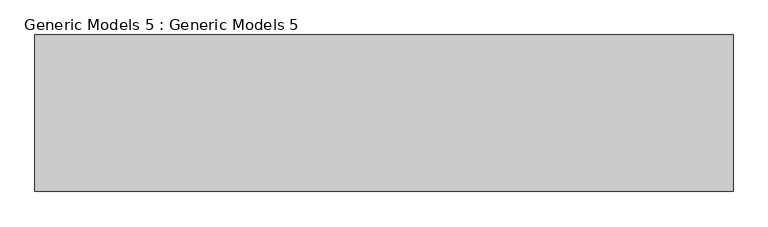
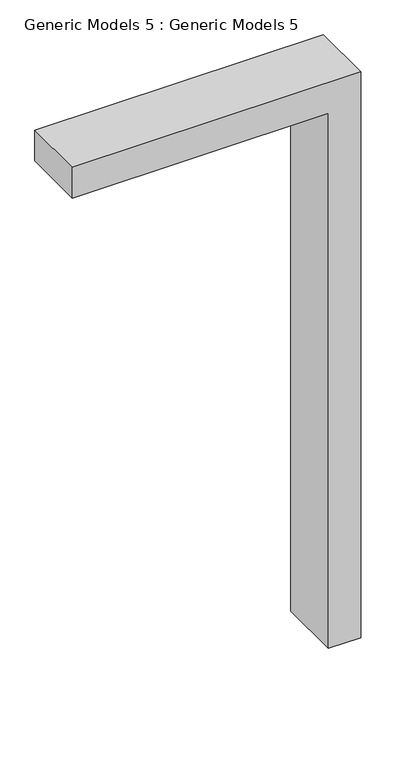
"""IFC4 building model written with IfcOpenShell, lengths in millimetres: proxy geometry, Generic Models 5 : Generic Models 5."""

from ifc_helpers import new_model, si_unit, frame, origin, place, context, project, spatial, polyline, outline, extrude, source, transform, mapped, element, save


def generic_models_5_generic_models_5_32b8a8a5(model_context):
    return source(origin(), model_context, "Body", "SweptSolid", [
        extrude(outline(polyline([(6019.1074387, -11546.1808371), (6019.1074387, -12905.5036722), (5866.7074387, -12905.5036722), (5866.7074387, -11698.5808371), (3200.4, -11698.5808371), (3200.4, -11546.1808371), (6019.1074387, -11546.1808371)])), frame((0.0, -11873.0453012, 0.0), z_axis=(0.0, 1.0, 0.0), x_axis=(0.0, 0.0, 1.0)), (0.0, 0.0, 1.0), 304.8),
    ])


if __name__ == "__main__":
    model = new_model("IFC4")
    model_context = context("Model", 3, world=origin())
    ifc_project = project(units=[si_unit("LENGTHUNIT", "METRE", prefix="MILLI")], contexts=[model_context])
    site = spatial("IfcSite", under=ifc_project)
    building = spatial("IfcBuilding", under=site)
    placement = place(None, origin())
    generic_models_5_generic_models_5_shape = generic_models_5_generic_models_5_32b8a8a5(model_context)
    element("IfcBuildingElementProxy", 1, Name="Generic Models 5 : Generic Models 5", ObjectType="Generic Models 5 : Generic Models 5", at=placement, inside=building, context=model_context, shape_type="MappedRepresentation", body=[
        mapped(generic_models_5_generic_models_5_shape, transform((0.0, 0.0, 0.0), x_axis=(1.0, 0.0, 0.0), y_axis=(0.0, 1.0, 0.0), z_axis=(0.0, 0.0, 1.0))),
    ])
    save(model, "model.ifc")

# Revit data of these elements
# Element 1 (IfcBuildingElementProxy, "Generic Models 5 : Generic Models 5")
#   Materials on its faces: "GREY COLOUR FRAME(1)"
# Materials
#   "GREY COLOUR FRAME(1)": class "Generic", colour RGB 120 120 120, transparency 0, Cost = 0
